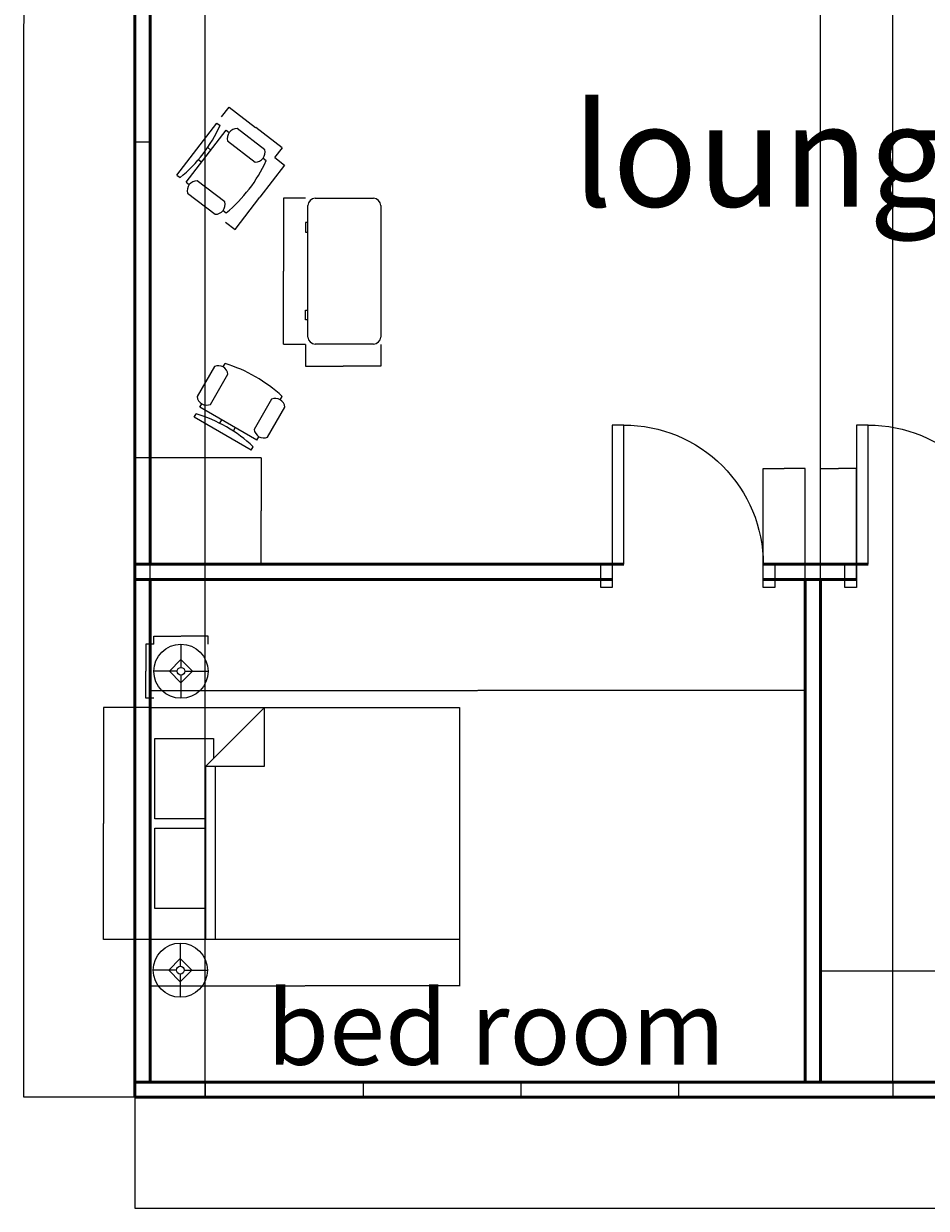
# Model space of a CAD drawing. Units: millimetres. Extents: x 756 to 17937, y 31 to 15590.
# Tile 1 of 6: x 1545 to 7469, y 31 to 7810. Entities that reach past the tile are written whole.
import ezdxf

# ---------------------------------------------------------------- set-up
doc = ezdxf.new("R2010")
doc.units = ezdxf.units.MM
for name, color, linetype, lineweight in [('A-ANNO-DIMS', 2, 'Continuous', 18), ('A-AREA-IDEN', 7, 'Continuous', 25), ('A-DOOR', 3, 'Continuous', 25), ('A-FURN', 8, 'Continuous', 18), ('A-GLAZ', 4, 'Continuous', 18), ('A-WALL', 7, 'Continuous', 50)]:
    doc.layers.add(name, color=color, linetype=linetype, lineweight=lineweight)
doc.styles.get("Standard").update_dxf_attribs({"font": 'arial.ttf'})
doc.dimstyles.get("Standard").update_dxf_attribs({"dimtxt": 0.18, "dimasz": 0.18, "dimexe": 0.18, "dimexo": 0.0625, "dimgap": 0.09, "dimtad": 0, "dimtih": 1, "dimtoh": 1, "dimdec": 4, "dimzin": 0, "dimdsep": 46, "dimtxsty": 'Standard', "dimcen": 0.09, "dimadec": 0, "dimazin": 0, "dimtfac": 1, "dimtdec": 4, "dimtofl": 0, "dimtmove": 0, "dimatfit": 3, "dimfxl": 1, "dimtolj": 1, "dimtzin": 0, "dimarcsym": 0})

# ---------------------------------------------------------------- blocks, each defined once
blk = doc.blocks.new('Bed - Queen')
for p, q in [((0, -80.00003), (0, 0)), ((0, 0), (59.99999, 0)), ((59.99999, 0), (59.99999, -80.00003)), ((7.99999, -1.2), (28.79998, -1.2)), ((7.99999, -14.4), (7.99999, -1.2)), ((28.79998, -1.2), (28.79998, -14.4)), ((31.19999, -1.2), (51.99999, -1.2)), ((31.19999, -14.4), (31.19999, -1.2)), ((51.99999, -1.2), (51.99999, -16.4)), ((0, -14.4), (44.8, -14.4)), ((59.99999, -29.6), (44.8, -14.4)), ((44.8, -14.4), (44.8, -29.6)), ((44.8, -16.8), (0, -16.8)), ((51.99999, -16.4), (46.79936, -16.4)), ((44.8, -29.6), (59.99999, -29.6)), ((59.99999, -80.00003), (0, -80.00003))]:
    blk.add_line(p, q)
blk = doc.blocks.new('Lamp - Table')
for p, q in [((0, 7), (0, 1)), ((-1, 0), (-7, 0)), ((0, 3), (-3, 0)), ((-3, 0), (0, -3)), ((3, 0), (0, 3)), ((0, -3), (3, 0)), ((1, 0), (7, 0)), ((0, -1), (0, -7))]:
    blk.add_line(p, q)
for radius in [7, 1]:
    blk.add_circle((0, 0), radius)
blk = doc.blocks.new('Chair - Desk')
for p, q in [((-8.5, 0), (-8.5, -1)), ((-8.5, 0), (8.5, 0)), ((8.5, 0), (8.5, -1)), ((-8.5, -3), (-8.5, -4)), ((-8.5, -3), (8.5, -3)), ((-2, -3), (-2, -1.9355)), ((2, -1.9576), (2, -3)), ((8.5, -3), (8.5, -4)), ((-10.5, -5), (-10.5, -14)), ((-6.5, -14), (-6.5, -5)), ((6.5, -5), (6.5, -14)), ((10.5, -14), (10.5, -5)), ((-8.5, -15), (-8.5, -16)), ((8.5, -15), (8.5, -16))]:
    blk.add_line(p, q)
for centre, radius, start, end in [((0, 34.625), 36.625, 256.5803, 283.4197), ((-8.5, -6.5), 2.5, 36.8699, 143.1301), ((8.5, -6.5), 2.5, 36.8699, 143.1301), ((-8.5, -12.5), 2.5, 216.8699, 323.1301), ((8.5, -12.5), 2.5, 216.8699, 323.1301), ((0, 19.625), 36.625, 256.5803, 283.4197)]:
    blk.add_arc(centre, radius, start, end)
blk = doc.blocks.new('Desk - 30 x 60 in.')
for p, q in [((-26.999995, 0), (26.999995, 0)), ((-29.999995, -27), (-29.999995, -3)), ((29.999995, -3), (29.999995, -27)), ((26.999995, -30), (-26.999995, -30)), ((-20.000005, -30), (-20.000005, -31)), ((-20.000005, -31), (-16.000005, -31)), ((-16.000005, -31), (-16.000005, -30)), ((15.999995, -31), (15.999995, -30)), ((19.999995, -31), (15.999995, -31)), ((19.999995, -30), (19.999995, -31))]:
    blk.add_line(p, q)
for centre, start, end in [((-26.499995, -3.5), 98.1301, 171.8699), ((26.499995, -3.5), 8.130102, 81.8699), ((-26.499995, -26.5), 188.1301, 261.8699), ((26.499995, -26.5), 278.1301, 351.8699)]:
    blk.add_arc(centre, 3.535534, start, end)
blk = doc.blocks.new('DOOR-SINGLE-914')
for p, q in [((76.2, 1066.8), (0, 1066.8)), ((0, 1066.8), (0, 914.4)), ((76.2, 914.4), (76.2, 1066.8)), ((1143, 1066.8), (1066.8, 1066.8)), ((1066.8, 1066.8), (1066.8, 914.4)), ((1143, 914.4), (1143, 1066.8)), ((0, 914.4), (76.2, 914.4)), ((76.2, 914.4), (152.4, 914.4)), ((76.2, 0), (76.2, 914.4)), ((152.4, 914.4), (152.4, 0)), ((1066.8, 914.4), (1143, 914.4)), ((152.4, 0), (76.2, 0))]:
    blk.add_line(p, q)
blk.add_arc((152.4, 914.4), 914.4, 270, 0)
blk = doc.blocks.new('WIN-2073')
for p, q in [((0, 100), (0, 0)), ((2072.9, 100), (0, 100)), ((2072.9, 0), (2072.9, 100)), ((0, 0), (2072.9, 0))]:
    blk.add_line(p, q)
blk = doc.blocks.new('*D21')
at = {"layer": 'A-ANNO-DIMS', "color": 0, "lineweight": -2, "transparency": 16777216}
for p, q in [((3193.5, 6930.8), (3257.2, 6882.2)), ((3256.9, 6882.1), (3095.2, 6670.6)), ((2933.1, 6458.7), (3094.9, 6670.2)), ((2869.5, 6507.2), (2933.1, 6458.5))]:
    blk.add_line(p, q, dxfattribs=at)
at = {"layer": 'A-ANNO-DIMS', "color": 0, "transparency": 16777216}
for points in [[(3256.9, 6882.1), (3257, 6882.1), (3257.1, 6882.3)], [(2933.1, 6458.7), (2933.1, 6458.7), (2933, 6458.6)]]:
    blk.add_solid(points, dxfattribs=at)
at = {"layer": 'Defpoints', "color": 0, "transparency": 16777216}
for p in [(3193.5, 6930.9), (3257.1, 6882.3), (2869.4, 6507.2)]:
    blk.add_point(p, dxfattribs=at)
at = {"layer": 'A-ANNO-DIMS', "color": 0, "transparency": 16777216, "insert": (3095, 6670.4), "char_height": 0.18, "attachment_point": 5}
blk.add_mtext('\\A1;CHAIR 533 TYP.', dxfattribs=at)
blk = doc.blocks.new('*D22')
at = {"layer": 'A-ANNO-DIMS', "color": 0, "lineweight": -2, "transparency": 16777216}
for p, q in [((2843.8, 7198.4), (2892.5, 7262)), ((2892.6, 7261.8), (3067, 7128.3)), ((3242, 6994.5), (3067.5, 7128)), ((3193.5, 6930.9), (3242.2, 6994.6))]:
    blk.add_line(p, q, dxfattribs=at)
at = {"layer": 'A-ANNO-DIMS', "color": 0, "transparency": 16777216}
for points in [[(2892.6, 7261.8), (2892.5, 7261.8), (2892.4, 7261.9)], [(3242, 6994.6), (3241.9, 6994.5), (3242.1, 6994.4)]]:
    blk.add_solid(points, dxfattribs=at)
at = {"layer": 'Defpoints', "color": 0, "transparency": 16777216}
for p in [(2892.4, 7261.9), (2843.8, 7198.4), (3193.5, 6930.9)]:
    blk.add_point(p, dxfattribs=at)
at = {"layer": 'A-ANNO-DIMS', "color": 0, "transparency": 16777216, "insert": (3067.3, 7128.2), "char_height": 0.18, "attachment_point": 5}
blk.add_mtext('\\A1;440 TYP.', dxfattribs=at)
blk = doc.blocks.new('*D23')
at = {"layer": 'A-ANNO-DIMS', "color": 0, "lineweight": -2, "transparency": 16777216}
for p, q in [((2398.9, 3735.6), (2398.9, 3789.1)), ((2399.1, 3788.9), (2575.7, 3788.9)), ((2754.3, 3788.9), (2577.6, 3788.9)), ((2754.5, 3735.6), (2754.5, 3789.1))]:
    blk.add_line(p, q, dxfattribs=at)
at = {"layer": 'A-ANNO-DIMS', "color": 0, "transparency": 16777216}
for points in [[(2399.1, 3788.9), (2399.1, 3788.9), (2398.9, 3788.9)], [(2754.3, 3788.9), (2754.3, 3788.9), (2754.5, 3788.9)]]:
    blk.add_solid(points, dxfattribs=at)
at = {"layer": 'Defpoints', "color": 0, "transparency": 16777216}
for p in [(2398.9, 3735.6), (2754.5, 3788.9), (2754.5, 3735.6)]:
    blk.add_point(p, dxfattribs=at)
at = {"layer": 'A-ANNO-DIMS', "color": 0, "transparency": 16777216, "insert": (2576.7, 3788.9), "char_height": 0.18, "attachment_point": 5}
blk.add_mtext('\\A1;LAMP 356 TYP.', dxfattribs=at)
blk = doc.blocks.new('*D24')
at = {"layer": 'A-ANNO-DIMS', "color": 0, "lineweight": -2, "transparency": 16777216}
for p, q in [((2398.8, 3735.6), (2345.4, 3735.6)), ((2345.5, 3735.4), (2345.5, 3557.9)), ((2345.5, 3380.1), (2345.5, 3557.6)), ((2398.8, 3380), (2345.4, 3380))]:
    blk.add_line(p, q, dxfattribs=at)
at = {"layer": 'A-ANNO-DIMS', "color": 0, "transparency": 16777216}
for points in [[(2345.5, 3735.4), (2345.6, 3735.4), (2345.5, 3735.6)], [(2345.5, 3380.1), (2345.6, 3380.1), (2345.5, 3380)]]:
    blk.add_solid(points, dxfattribs=at)
at = {"layer": 'Defpoints', "color": 0, "transparency": 16777216}
for p in [(2345.5, 3735.6), (2398.9, 3735.6), (2398.9, 3380)]:
    blk.add_point(p, dxfattribs=at)
at = {"layer": 'A-ANNO-DIMS', "color": 0, "transparency": 16777216, "insert": (2345.5, 3557.8), "char_height": 0.18, "attachment_point": 5}
blk.add_mtext('\\A1;356 TYP.', dxfattribs=at)
blk = doc.blocks.new('*D25')
at = {"layer": 'A-ANNO-DIMS', "color": 0, "lineweight": -2, "transparency": 16777216}
for p, q in [((2374.1, 1795.4), (2374.1, 1490.5)), ((4406.1, 1795.4), (4406.1, 1490.5)), ((2374.3, 1490.7), (3389, 1490.7)), ((4405.9, 1490.7), (3391.2, 1490.7))]:
    blk.add_line(p, q, dxfattribs=at)
at = {"layer": 'A-ANNO-DIMS', "color": 0, "transparency": 16777216}
for points in [[(2374.3, 1490.7), (2374.3, 1490.6), (2374.1, 1490.7)], [(4405.9, 1490.7), (4405.9, 1490.6), (4406.1, 1490.7)]]:
    blk.add_solid(points, dxfattribs=at)
at = {"layer": 'Defpoints', "color": 0, "transparency": 16777216}
for p in [(2374.1, 1795.5), (4406.1, 1795.5), (2374.1, 1490.7)]:
    blk.add_point(p, dxfattribs=at)
at = {"layer": 'A-ANNO-DIMS', "color": 0, "transparency": 16777216, "insert": (3390.1, 1490.7), "char_height": 0.18, "attachment_point": 5}
blk.add_mtext('\\A1;QUEEN BED 2032', dxfattribs=at)
blk = doc.blocks.new('*D26')
at = {"layer": 'A-ANNO-DIMS', "color": 0, "lineweight": -2, "transparency": 16777216}
for p, q in [((2374.1, 3319.5), (2069.1, 3319.5)), ((2069.3, 3319.3), (2069.3, 2557.6)), ((2069.3, 1795.6), (2069.3, 2557.3)), ((2374.1, 1795.5), (2069.1, 1795.5))]:
    blk.add_line(p, q, dxfattribs=at)
at = {"layer": 'A-ANNO-DIMS', "color": 0, "transparency": 16777216}
for points in [[(2069.3, 3319.3), (2069.3, 3319.3), (2069.3, 3319.5)], [(2069.3, 1795.6), (2069.3, 1795.6), (2069.3, 1795.5)]]:
    blk.add_solid(points, dxfattribs=at)
at = {"layer": 'Defpoints', "color": 0, "transparency": 16777216}
for p in [(2069.3, 3319.5), (2374.1, 3319.5), (2374.1, 1795.5)]:
    blk.add_point(p, dxfattribs=at)
at = {"layer": 'A-ANNO-DIMS', "color": 0, "transparency": 16777216, "insert": (2069.3, 2557.5), "char_height": 0.18, "attachment_point": 5}
blk.add_mtext('\\A1;1524', dxfattribs=at)
blk = doc.blocks.new('*D33')
at = {"layer": 'A-ANNO-DIMS', "color": 0, "lineweight": -2, "transparency": 16777216}
for p, q in [((3393.3, 6664.7), (3249.2, 6664.7)), ((3249.4, 6664.6), (3249.4, 6184.8)), ((3249.4, 5704.7), (3249.4, 6184.5)), ((3393.3, 5704.5), (3249.2, 5704.5))]:
    blk.add_line(p, q, dxfattribs=at)
at = {"layer": 'A-ANNO-DIMS', "color": 0, "transparency": 16777216}
for points in [[(3249.3, 6664.6), (3249.4, 6664.6), (3249.4, 6664.7)], [(3249.3, 5704.7), (3249.4, 5704.7), (3249.4, 5704.5)]]:
    blk.add_solid(points, dxfattribs=at)
at = {"layer": 'Defpoints', "color": 0, "transparency": 16777216}
for p in [(3393.4, 6664.7), (3249.4, 5704.5), (3393.4, 5704.5)]:
    blk.add_point(p, dxfattribs=at)
at = {"layer": 'A-ANNO-DIMS', "color": 0, "transparency": 16777216, "insert": (3249.4, 6184.6), "char_height": 0.18, "attachment_point": 5}
blk.add_mtext('\\A1;DESK 960', dxfattribs=at)
blk = doc.blocks.new('*D34')
at = {"layer": 'A-ANNO-DIMS', "color": 0, "lineweight": -2, "transparency": 16777216}
for p, q in [((3393.4, 5704.5), (3393.4, 5560.3)), ((3889.5, 5704.5), (3889.5, 5560.3)), ((3393.6, 5560.5), (3641.1, 5560.5)), ((3889.3, 5560.5), (3641.7, 5560.5))]:
    blk.add_line(p, q, dxfattribs=at)
at = {"layer": 'A-ANNO-DIMS', "color": 0, "transparency": 16777216}
for points in [[(3393.6, 5560.5), (3393.6, 5560.5), (3393.4, 5560.5)], [(3889.3, 5560.5), (3889.3, 5560.5), (3889.5, 5560.5)]]:
    blk.add_solid(points, dxfattribs=at)
at = {"layer": 'Defpoints', "color": 0, "transparency": 16777216}
for p in [(3393.4, 5704.5), (3889.5, 5704.5), (3889.5, 5560.5)]:
    blk.add_point(p, dxfattribs=at)
at = {"layer": 'A-ANNO-DIMS', "color": 0, "transparency": 16777216, "insert": (3641.4, 5560.5), "char_height": 0.18, "attachment_point": 5}
blk.add_mtext('\\A1;496', dxfattribs=at)
blk = doc.blocks.new('*D43')
at = {"layer": 'A-ANNO-DIMS', "color": 0, "lineweight": -2, "transparency": 16777216}
for p, q in [((16790.9, 2160.1), (16790.9, 30.8)), ((2274.1, 760.1), (2274.1, 30.8)), ((2274.3, 30.9), (9532.1, 30.9)), ((16790.7, 30.9), (9532.9, 30.9))]:
    blk.add_line(p, q, dxfattribs=at)
at = {"layer": 'A-ANNO-DIMS', "color": 0, "transparency": 16777216}
for points in [[(2274.3, 31), (2274.3, 30.9), (2274.1, 30.9)], [(16790.7, 31), (16790.7, 30.9), (16790.9, 30.9)]]:
    blk.add_solid(points, dxfattribs=at)
at = {"layer": 'Defpoints', "color": 0, "transparency": 16777216}
for p in [(16790.9, 2160.2), (2274.1, 760.2), (16790.9, 30.9)]:
    blk.add_point(p, dxfattribs=at)
at = {"layer": 'A-ANNO-DIMS', "color": 0, "transparency": 16777216, "insert": (9532.5, 30.9), "char_height": 0.18, "attachment_point": 5}
blk.add_mtext('\\A1;14517', dxfattribs=at)
blk = doc.blocks.new('*D44')
at = {"layer": 'A-ANNO-DIMS', "color": 0, "lineweight": -2, "transparency": 16777216}
for p, q in [((2274.1, 14860.2), (1544.7, 14860.2)), ((1544.9, 14860), (1544.9, 7810.4)), ((1544.9, 760.4), (1544.9, 7810)), ((2274.1, 760.2), (1544.7, 760.2))]:
    blk.add_line(p, q, dxfattribs=at)
at = {"layer": 'A-ANNO-DIMS', "color": 0, "transparency": 16777216}
for points in [[(1544.8, 14860), (1544.9, 14860), (1544.9, 14860.2)], [(1544.8, 760.4), (1544.9, 760.4), (1544.9, 760.2)]]:
    blk.add_solid(points, dxfattribs=at)
at = {"layer": 'Defpoints', "color": 0, "transparency": 16777216}
for p in [(1544.9, 14860.2), (2274.1, 14860.2), (2274.1, 760.2)]:
    blk.add_point(p, dxfattribs=at)
at = {"layer": 'A-ANNO-DIMS', "color": 0, "transparency": 16777216, "insert": (1544.9, 7810.2), "char_height": 0.18, "attachment_point": 5}
blk.add_mtext('\\A1;14100', dxfattribs=at)
blk = doc.blocks.new('*D45')
at = {"layer": 'A-ANNO-DIMS', "color": 0, "lineweight": -2, "transparency": 16777216}
for p, q in [((2374.1, 4160.1), (2374.1, 3430.8)), ((6674.1, 4160.1), (6674.1, 3430.8)), ((2374.3, 3430.9), (4523.8, 3430.9)), ((6673.9, 3430.9), (4524.5, 3430.9))]:
    blk.add_line(p, q, dxfattribs=at)
at = {"layer": 'A-ANNO-DIMS', "color": 0, "transparency": 16777216}
for points in [[(2374.3, 3431), (2374.3, 3430.9), (2374.1, 3430.9)], [(6673.9, 3431), (6673.9, 3430.9), (6674.1, 3430.9)]]:
    blk.add_solid(points, dxfattribs=at)
at = {"layer": 'Defpoints', "color": 0, "transparency": 16777216}
for p in [(2374.1, 4160.2), (6674.1, 4160.2), (2374.1, 3430.9)]:
    blk.add_point(p, dxfattribs=at)
at = {"layer": 'A-ANNO-DIMS', "color": 0, "transparency": 16777216, "insert": (4524.1, 3430.9), "char_height": 0.18, "attachment_point": 5}
blk.add_mtext('\\A1;4300', dxfattribs=at)
blk = doc.blocks.new('*D46')
at = {"layer": 'A-ANNO-DIMS', "color": 0, "lineweight": -2, "transparency": 16777216}
for p, q in [((6774.1, 860.2), (6774.1, 1589.6)), ((6774.3, 1589.4), (8923.8, 1589.4)), ((11073.9, 1589.4), (8924.5, 1589.4)), ((11074.1, 860.2), (11074.1, 1589.6))]:
    blk.add_line(p, q, dxfattribs=at)
at = {"layer": 'A-ANNO-DIMS', "color": 0, "transparency": 16777216}
for points in [[(6774.3, 1589.5), (6774.3, 1589.4), (6774.1, 1589.4)], [(11073.9, 1589.5), (11073.9, 1589.4), (11074.1, 1589.4)]]:
    blk.add_solid(points, dxfattribs=at)
at = {"layer": 'Defpoints', "color": 0, "transparency": 16777216}
for p in [(11074.1, 1589.4), (6774.1, 860.2), (11074.1, 860.2)]:
    blk.add_point(p, dxfattribs=at)
at = {"layer": 'A-ANNO-DIMS', "color": 0, "transparency": 16777216, "insert": (8924.1, 1589.4), "char_height": 0.18, "attachment_point": 5}
blk.add_mtext('\\A1;4300', dxfattribs=at)
blk = doc.blocks.new('*D63')
at = {"layer": 'A-ANNO-DIMS', "color": 0, "lineweight": -2, "transparency": 16777216}
for p, q in [((2374.1, 860.2), (2374.1, 15589.6)), ((2374.3, 15589.4), (2554.6, 15589.4)), ((2735.7, 15589.4), (2555.4, 15589.4)), ((2735.9, 760.2), (2735.9, 15589.6))]:
    blk.add_line(p, q, dxfattribs=at)
at = {"layer": 'A-ANNO-DIMS', "color": 0, "transparency": 16777216}
for points in [[(2374.3, 15589.5), (2374.3, 15589.4), (2374.1, 15589.4)], [(2735.7, 15589.5), (2735.7, 15589.4), (2735.9, 15589.4)]]:
    blk.add_solid(points, dxfattribs=at)
at = {"layer": 'Defpoints', "color": 0, "transparency": 16777216}
for p in [(2735.9, 15589.4), (2374.1, 860.2), (2735.9, 760.2)]:
    blk.add_point(p, dxfattribs=at)
at = {"layer": 'A-ANNO-DIMS', "color": 0, "transparency": 16777216, "insert": (2555, 15589.4), "char_height": 0.18, "attachment_point": 5}
blk.add_mtext('\\A1;361.8', dxfattribs=at)
blk = doc.blocks.new('*D64')
at = {"layer": 'A-ANNO-DIMS', "color": 0, "lineweight": -2, "transparency": 16777216}
for p, q in [((6774.1, 860.2), (6774.1, 15589.6)), ((6774.3, 15589.4), (7011.6, 15589.4)), ((7249.8, 15589.4), (7012.4, 15589.4)), ((7250, 860.2), (7250, 15589.6))]:
    blk.add_line(p, q, dxfattribs=at)
at = {"layer": 'A-ANNO-DIMS', "color": 0, "transparency": 16777216}
for points in [[(6774.3, 15589.5), (6774.3, 15589.4), (6774.1, 15589.4)], [(7249.8, 15589.5), (7249.8, 15589.4), (7250, 15589.4)]]:
    blk.add_solid(points, dxfattribs=at)
at = {"layer": 'Defpoints', "color": 0, "transparency": 16777216}
for p in [(7250, 15589.4), (6774.1, 860.2), (7250, 860.2)]:
    blk.add_point(p, dxfattribs=at)
at = {"layer": 'A-ANNO-DIMS', "color": 0, "transparency": 16777216, "insert": (7012, 15589.4), "char_height": 0.18, "attachment_point": 5}
blk.add_mtext('\\A1;475.9', dxfattribs=at)
blk = doc.blocks.new('*D66')
at = {"layer": 'A-ANNO-DIMS', "color": 0, "lineweight": -2, "transparency": 16777216}
for p, q in [((2374.2, 4960.3), (3103.5, 4960.3)), ((3103.4, 4960.2), (3103.4, 4610.4)), ((3103.4, 4260.4), (3103.4, 4610.1)), ((2374.2, 4260.2), (3103.5, 4260.2))]:
    blk.add_line(p, q, dxfattribs=at)
at = {"layer": 'A-ANNO-DIMS', "color": 0, "transparency": 16777216}
for points in [[(3103.3, 4960.2), (3103.4, 4960.2), (3103.4, 4960.3)], [(3103.3, 4260.4), (3103.4, 4260.4), (3103.4, 4260.2)]]:
    blk.add_solid(points, dxfattribs=at)
at = {"layer": 'Defpoints', "color": 0, "transparency": 16777216}
for p in [(2374.1, 4960.3), (2374.1, 4260.2), (3103.4, 4260.2)]:
    blk.add_point(p, dxfattribs=at)
at = {"layer": 'A-ANNO-DIMS', "color": 0, "transparency": 16777216, "insert": (3103.4, 4610.3), "char_height": 0.18, "attachment_point": 5}
blk.add_mtext('\\A1;700.2', dxfattribs=at)
blk = doc.blocks.new('*D75')
at = {"layer": 'A-ANNO-DIMS', "color": 0, "lineweight": -2, "transparency": 16777216}
for p, q in [((6398.6, 4160.2), (6398.6, 4889.6)), ((6398.8, 4889.4), (6536, 4889.4)), ((6673.9, 4889.4), (6536.7, 4889.4)), ((6674.1, 4160.2), (6674.1, 4889.6))]:
    blk.add_line(p, q, dxfattribs=at)
at = {"layer": 'A-ANNO-DIMS', "color": 0, "transparency": 16777216}
for points in [[(6398.8, 4889.5), (6398.8, 4889.4), (6398.6, 4889.4)], [(6673.9, 4889.5), (6673.9, 4889.4), (6674.1, 4889.4)]]:
    blk.add_solid(points, dxfattribs=at)
at = {"layer": 'Defpoints', "color": 0, "transparency": 16777216}
for p in [(6674.1, 4889.4), (6398.6, 4160.2), (6674.1, 4160.2)]:
    blk.add_point(p, dxfattribs=at)
at = {"layer": 'A-ANNO-DIMS', "color": 0, "transparency": 16777216, "insert": (6536.4, 4889.4), "char_height": 0.18, "attachment_point": 5}
blk.add_mtext('\\A1;275.5', dxfattribs=at)
blk = doc.blocks.new('*D76')
at = {"layer": 'A-ANNO-DIMS', "color": 0, "lineweight": -2, "transparency": 16777216}
for p, q in [((6774.1, 4160.2), (6774.1, 4889.6)), ((6774.3, 4889.4), (6892.4, 4889.4)), ((7011.4, 4889.4), (6893.2, 4889.4)), ((7011.5, 4160.2), (7011.5, 4889.6))]:
    blk.add_line(p, q, dxfattribs=at)
at = {"layer": 'A-ANNO-DIMS', "color": 0, "transparency": 16777216}
for points in [[(6774.3, 4889.5), (6774.3, 4889.4), (6774.1, 4889.4)], [(7011.4, 4889.5), (7011.4, 4889.4), (7011.5, 4889.4)]]:
    blk.add_solid(points, dxfattribs=at)
at = {"layer": 'Defpoints', "color": 0, "transparency": 16777216}
for p in [(7011.5, 4889.4), (6774.1, 4160.2), (7011.5, 4160.2)]:
    blk.add_point(p, dxfattribs=at)
at = {"layer": 'A-ANNO-DIMS', "color": 0, "transparency": 16777216, "insert": (6892.8, 4889.4), "char_height": 0.18, "attachment_point": 5}
blk.add_mtext('\\A1;237.4', dxfattribs=at)

msp = doc.modelspace()

# ---------------------------------------------------------------- linework, layer by layer
at = {"layer": 'A-WALL'}
for p, q in [((2274.114, 4260.181), (2274.114, 9560.181)), ((2374.114, 9460.181), (2374.114, 4260.181)), ((2274.114, 4160.181), (2274.114, 4260.181)), ((2274.114, 4260.181), (5484.189, 4260.181)), ((6398.589, 4260.181), (7087.731, 4260.181)), ((2274.114, 860.181), (2274.114, 4160.181)), ((2274.114, 4160.181), (5407.989, 4160.181)), ((5407.989, 4160.181), (2274.114, 4160.181)), ((2374.114, 4160.181), (2374.114, 860.181)), ((6574.114, 4160.181), (6398.589, 4160.181)), ((6398.589, 4160.181), (7011.531, 4160.181)), ((6674.114, 860.181), (6674.114, 4160.181)), ((6774.114, 4160.181), (6774.114, 860.181)), ((7011.531, 4160.181), (6774.114, 4160.181)), ((2374.114, 860.181), (2274.114, 860.181)), ((2274.114, 760.181), (2274.114, 860.181)), ((2374.114, 860.181), (6674.114, 860.181)), ((6574.114, 860.181), (6674.114, 860.181)), ((6774.114, 860.181), (6574.114, 860.181)), ((6674.114, 860.181), (10974.114, 860.181)), ((6874.114, 760.181), (2274.114, 760.181)), ((11174.114, 760.181), (6874.114, 760.181))]:
    msp.add_line(p, q, dxfattribs=at)

# ---------------------------------------------------------------- block references
at = {"layer": 'A-DOOR', "extrusion": (0, 0, -1), "zscale": -1, "rotation": 180}
for p in [(-5331.789, 5174.581), (-6935.331, 5174.581)]:
    msp.add_blockref('DOOR-SINGLE-914', p, dxfattribs=at)
at = {"layer": 'A-FURN'}
for name, p, xscale, yscale, zscale, rotation in [('Chair - Desk', (2681.769, 6986.513), 25.4, 25.4, 25.4, 52.58843820834264), ('Desk - 30 x 60 in.', (3889.482, 6184.637), 16.00322632039982, 16.00322632039982, 16.00322632039982, 270), ('Chair - Desk', (2850.612, 5117.872), 25.4, 25.4, 25.4, 150.0574916853524), ('Bed - Queen', (2374.114, 1795.454), 25.4, 25.4, 25.4, 90)]:
    msp.add_blockref(name, p, dxfattribs=dict(at, xscale=xscale, yscale=yscale, zscale=zscale, rotation=rotation))
at = {"layer": 'A-FURN', "xscale": 25.4, "yscale": 25.4, "zscale": 25.4}
for p in [(2576.671, 3557.764), (2572.491, 1594.771)]:
    msp.add_blockref('Lamp - Table', p, dxfattribs=at)
at = {"layer": 'A-GLAZ', "rotation": 90.00000000000003}
msp.add_blockref('WIN-2073', (2374.113, 4960.332), dxfattribs=at)
at = {"layer": 'A-GLAZ'}
for p in [(2735.923, 760.181), (3772.375, 760.181), (7249.967, 760.181)]:
    msp.add_blockref('WIN-2073', p, dxfattribs=at)

# ---------------------------------------------------------------- texts
at = {"layer": 'A-AREA-IDEN', "attachment_point": 1}
for s, width, gutter_width, insert, char_height in [('lounge', 8015.31461, 3380.597, (5146.97, 7285.035), 676.1193), ('bed room', 9167.49825, 2429.33, (3139.251, 1459.237), 485.8659)]:
    msp.add_mtext_dynamic_manual_height_columns(s, width=width, gutter_width=gutter_width, heights=[0], dxfattribs=dict(at, insert=insert, char_height=char_height))

# ---------------------------------------------------------------- dimensions: what is measured, and where the dimension line sits
at = {"layer": 'A-ANNO-DIMS'}
for base, p1, p2, override, picture, middle in [((2735.923, 15589.431), (2374.114, 860.181), (2735.923, 760.181), {"dimdec": 1, "dimlfac": 1, "dimrnd": 0, "dimzin": 0, "dimdsep": 46, "dimlunit": 2}, '*D63', (2555.018, 15589.431)), ((7249.967, 15589.431), (6774.114, 860.181), (7249.967, 860.181), {"dimdec": 1, "dimlfac": 1, "dimrnd": 0, "dimzin": 0, "dimdsep": 46, "dimlunit": 2}, '*D64', (7012.041, 15589.431)), ((3889.482, 5560.511), (3393.382, 5704.54), (3889.482, 5704.54), {"dimdec": 0, "dimlfac": 1, "dimrnd": 0, "dimzin": 0, "dimdsep": 46, "dimlunit": 2}, '*D34', (3641.432, 5560.511)), ((6674.114, 4889.431), (6398.589, 4160.181), (6674.114, 4160.181), {"dimdec": 1, "dimlfac": 1, "dimrnd": 0, "dimzin": 0, "dimdsep": 46, "dimlunit": 2}, '*D75', (6536.351, 4889.431)), ((7011.531, 4889.431), (6774.114, 4160.181), (7011.531, 4160.181), {"dimdec": 1, "dimlfac": 1, "dimrnd": 0, "dimzin": 0, "dimdsep": 46, "dimlunit": 2}, '*D76', (6892.822, 4889.431)), ((16790.928, 30.931), (2274.114, 760.181), (16790.928, 2160.181), {"dimdec": 0, "dimlfac": 1, "dimrnd": 0, "dimzin": 0, "dimdsep": 46, "dimlunit": 2}, '*D43', (9532.521, 30.931)), ((11074.114, 1589.431), (6774.114, 860.181), (11074.114, 860.181), {"dimdec": 0, "dimlfac": 1, "dimrnd": 0, "dimzin": 0, "dimdsep": 46, "dimlunit": 2}, '*D46', (8924.114, 1589.431))]:
    dim = msp.add_linear_dim(base=base, p1=p1, p2=p2, dimstyle='Standard', override=override, dxfattribs=at)
    dim.commit()
    dim.dimension.update_dxf_attribs({"geometry": picture, "text_midpoint": middle})
for base, p1, p2, angle, override, picture, middle in [((1544.864, 14860.181), (2274.114, 760.181), (2274.114, 14860.181), 90, {"dimdec": 0, "dimlfac": 1, "dimrnd": 0, "dimzin": 0, "dimdsep": 46, "dimlunit": 2}, '*D44', (1544.864, 7810.181)), ((3103.364, 4260.181), (2374.114, 4960.332), (2374.114, 4260.181), 270, {"dimdec": 1, "dimlfac": 1, "dimrnd": 0, "dimzin": 0, "dimdsep": 46, "dimlunit": 2}, '*D66', (3103.364, 4610.256)), ((2374.114, 3430.931), (6674.114, 4160.181), (2374.114, 4160.181), 180, {"dimdec": 0, "dimlfac": 1, "dimrnd": 0, "dimzin": 0, "dimdsep": 46, "dimlunit": 2}, '*D45', (4524.114, 3430.931)), ((2069.314, 3319.454), (2374.114, 1795.454), (2374.114, 3319.454), 90, {"dimdec": 0, "dimlfac": 1, "dimrnd": 0, "dimzin": 0, "dimdsep": 46, "dimlunit": 2}, '*D26', (2069.314, 2557.454))]:
    dim = msp.add_linear_dim(base=base, p1=p1, p2=p2, angle=angle, dimstyle='Standard', override=override, dxfattribs=at)
    dim.commit()
    dim.dimension.update_dxf_attribs({"geometry": picture, "text_midpoint": middle})
for base, p1, p2, angle, text, picture, middle in [((2892.408, 7261.902), (3193.499, 6930.873), (2843.799, 7198.351), 142.5884382, '<> TYP.', '*D22', (3067.258, 7128.163)), ((3257.05, 6882.264), (2869.439, 6507.198), (3193.499, 6930.873), 52.5884382, 'CHAIR <> TYP.', '*D21', (3095.021, 6670.426)), ((3249.353, 5704.54), (3393.382, 6664.733), (3393.382, 5704.54), 270, 'DESK <>', '*D33', (3249.353, 6184.637)), ((2345.531, 3735.564), (2398.871, 3379.964), (2398.871, 3735.564), 90, '<> TYP.', '*D24', (2345.531, 3557.764)), ((2374.114, 1490.654), (4406.114, 1795.454), (2374.114, 1795.454), 180, 'QUEEN BED <>', '*D25', (3390.114, 1490.654))]:
    dim = msp.add_linear_dim(base=base, p1=p1, p2=p2, angle=angle, text=text, dimstyle='Standard', override={"dimdec": 0, "dimlfac": 1, "dimrnd": 0, "dimzin": 0, "dimdsep": 46, "dimlunit": 2}, dxfattribs=at)
    dim.commit()
    dim.dimension.update_dxf_attribs({"geometry": picture, "text_midpoint": middle})
dim = msp.add_linear_dim(base=(2754.471, 3788.904), p1=(2398.871, 3735.564), p2=(2754.471, 3735.564), text='LAMP <> TYP.', dimstyle='Standard', override={"dimdec": 0, "dimlfac": 1, "dimrnd": 0, "dimzin": 0, "dimdsep": 46, "dimlunit": 2}, dxfattribs=at)
dim.commit()
dim.dimension.update_dxf_attribs({"geometry": '*D23', "text_midpoint": (2576.671, 3788.904)})

doc.saveas('drawing.dxf')
